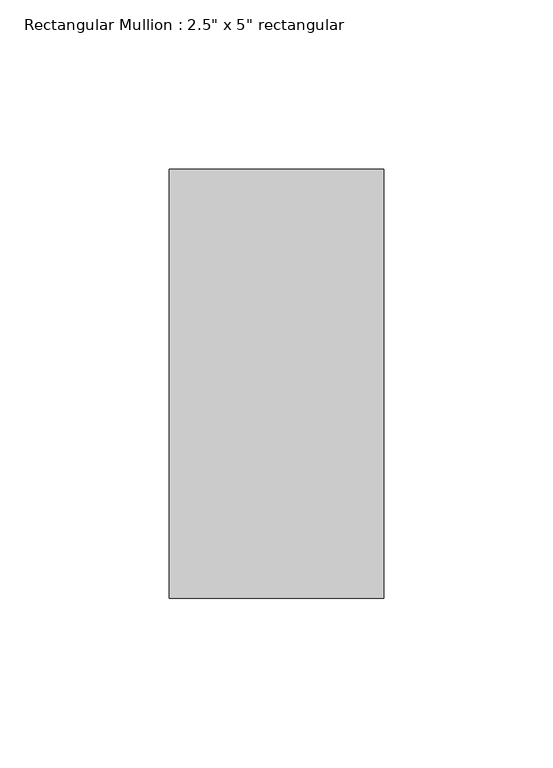
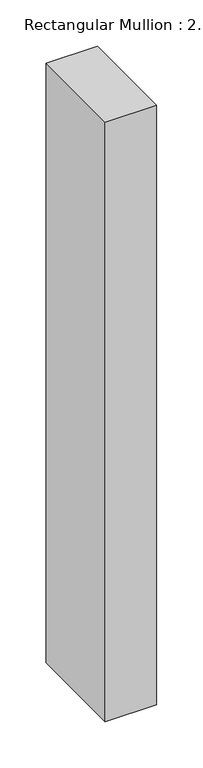
"""IFC4 building model written with IfcOpenShell, lengths in millimetres: member geometry."""

from ifc_helpers import new_model, si_unit, frame, origin, place, context, project, spatial, polyline, outline, extrude, source, transform, mapped, element, save


def member_429f6687(model_context):
    return source(origin(), model_context, "Body", "SweptSolid", [
        extrude(outline(polyline([(0.0, 63.5), (0.0, -63.5), (-63.5, -63.5), (-63.5, 63.5), (0.0, 63.5)])), frame((0.0, 0.0, -787.4), z_axis=(0.0, 0.0, 1.0), x_axis=(1.0, 0.0, 0.0)), (0.0, 0.0, 1.0), 787.4),
    ])


if __name__ == "__main__":
    model = new_model("IFC4")
    model_context = context("Model", 3, world=origin())
    ifc_project = project(units=[si_unit("LENGTHUNIT", "METRE", prefix="MILLI")], contexts=[model_context])
    site = spatial("IfcSite", under=ifc_project)
    building = spatial("IfcBuilding", under=site)
    placement = place(None, origin())
    member_shape = member_429f6687(model_context)
    element("IfcMember", 1, ObjectType="Rectangular Mullion : 2.5\" x 5\" rectangular", at=placement, inside=building, context=model_context, shape_type="MappedRepresentation", body=[
        mapped(member_shape, transform((0.0, 0.0, 0.0), x_axis=(1.0, 0.0, 0.0), y_axis=(0.0, 1.0, 0.0), z_axis=(0.0, 0.0, 1.0))),
    ])
    save(model, "model.ifc")

# Revit data of these elements
# Type "Rectangular Mullion : 2.5\" x 5\" rectangular"
#   built-in parameter 1007304 = 0.416667 (stored number, unit not read)
#   built-in parameter 1007301 = 0.104167 (stored number, unit not read)
#   built-in parameter 1007300 = 0.104167 (stored number, unit not read)
# Element 1 (IfcMember, "Rectangular Mullion : 2.5\" x 5\" rectangular")
#   Materials on its faces: "BLACK MATERIAL"
# Materials
#   "BLACK MATERIAL": class "Generic", colour RGB 120 120 120, transparency 0, Cost = 0
